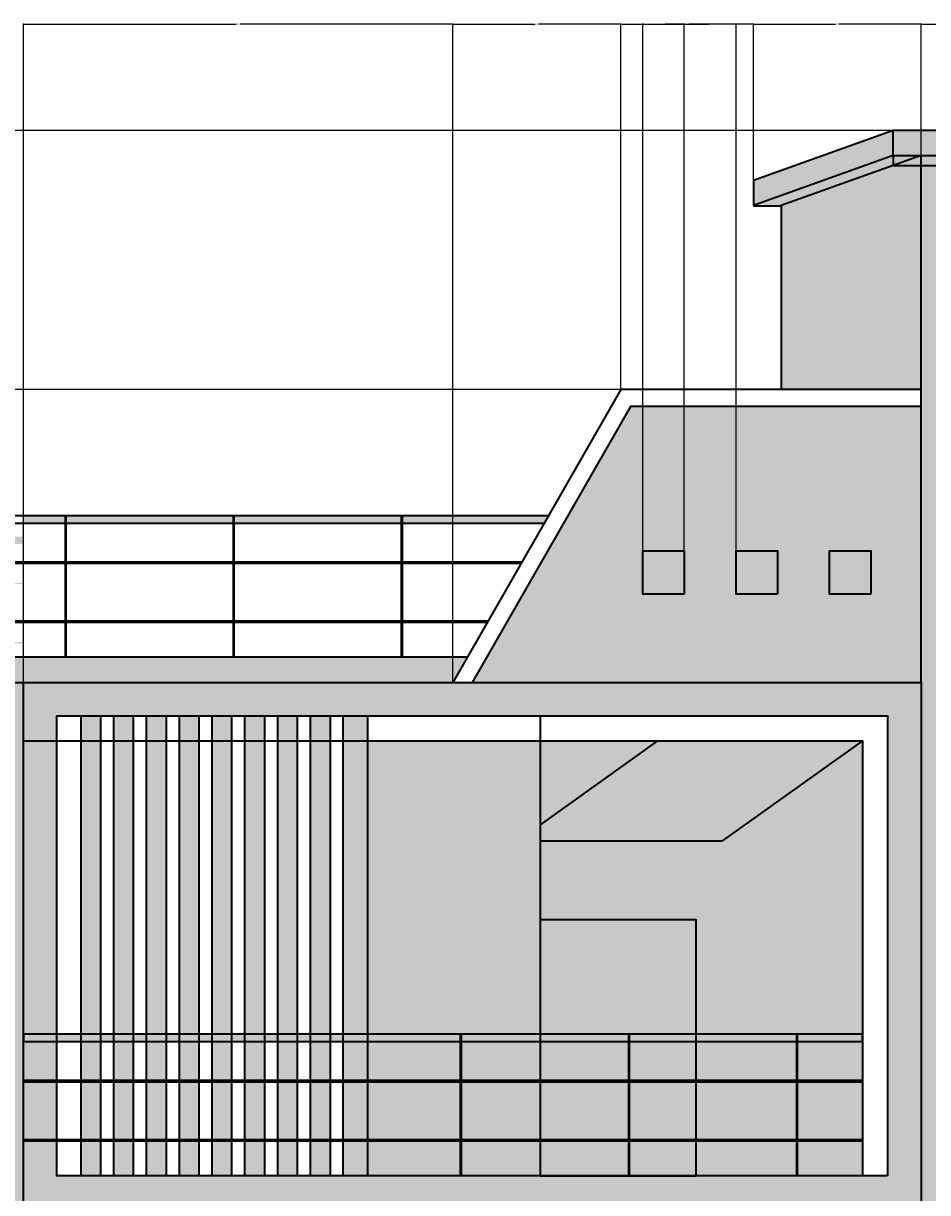
# Model space of a CAD drawing. Units: feet. Extents: x 2415 to 6174, y 866 to 1295.
# Tile 3 of 9: x 3364 to 3580, y 1016 to 1295. Entities that reach past the tile are written whole.
import ezdxf

# ---------------------------------------------------------------- set-up
doc = ezdxf.new("R2010")
doc.units = ezdxf.units.FT
for name, color, linetype, lineweight in [('A-ANNO-DIMS', 2, 'Continuous', 18), ('A-ELEV', 7, 'Continuous', 35), ('A-ELEV-PATT', 8, 'Continuous', 13)]:
    doc.layers.add(name, color=color, linetype=linetype, lineweight=lineweight)
doc.styles.get("Standard").update_dxf_attribs({"font": 'arial.ttf'})
doc.dimstyles.get("Standard").update_dxf_attribs({"dimtxt": 0.18, "dimasz": 0.18, "dimexe": 0.18, "dimexo": 0.0625, "dimgap": 0.09, "dimtad": 0, "dimtih": 1, "dimtoh": 1, "dimdec": 1, "dimzin": 0, "dimdsep": 46, "dimlunit": 3, "dimtxsty": 'Standard', "dimcen": 0.09, "dimadec": 0, "dimazin": 0, "dimtfac": 1, "dimtdec": 1, "dimtofl": 0, "dimtmove": 0, "dimatfit": 3, "dimfxl": 1, "dimtolj": 1, "dimtzin": 0, "dimarcsym": 0})

# ---------------------------------------------------------------- blocks, each defined once
blk = doc.blocks.new('*D63')
at = {"layer": 'A-ANNO-DIMS', "color": 0, "lineweight": -2, "transparency": 16777216}
for p, q in [((3363.87, 1137.66), (3363.87, 1295.18)), ((3364.05, 1295), (3414.78, 1295)), ((3466.42, 1295), (3415.69, 1295)), ((3466.6, 1137.66), (3466.6, 1295.18))]:
    blk.add_line(p, q, dxfattribs=at)
at = {"layer": 'A-ANNO-DIMS', "color": 0, "transparency": 16777216}
for points in [[(3364.05, 1295.03), (3364.05, 1294.97), (3363.87, 1295)], [(3466.42, 1295.03), (3466.42, 1294.97), (3466.6, 1295)]]:
    blk.add_solid(points, dxfattribs=at)
at = {"layer": 'Defpoints', "color": 0, "transparency": 16777216}
for p in [(3466.6, 1295), (3363.87, 1137.6), (3466.6, 1137.6)]:
    blk.add_point(p, dxfattribs=at)
at = {"layer": 'A-ANNO-DIMS', "color": 0, "transparency": 16777216, "insert": (3415.23, 1295), "char_height": 0.18, "attachment_point": 5}
blk.add_mtext('\\A1;102.73', dxfattribs=at)
blk = doc.blocks.new('*D64')
at = {"layer": 'A-ANNO-DIMS', "color": 0, "lineweight": -2, "transparency": 16777216}
for p, q in [((3466.6, 1137.66), (3466.6, 1295.18)), ((3466.78, 1295), (3486.3, 1295)), ((3506.61, 1295), (3487.09, 1295)), ((3506.79, 1207.66), (3506.79, 1295.18))]:
    blk.add_line(p, q, dxfattribs=at)
at = {"layer": 'A-ANNO-DIMS', "color": 0, "transparency": 16777216}
for points in [[(3466.78, 1295.03), (3466.78, 1294.97), (3466.6, 1295)], [(3506.61, 1295.03), (3506.61, 1294.97), (3506.79, 1295)]]:
    blk.add_solid(points, dxfattribs=at)
at = {"layer": 'Defpoints', "color": 0, "transparency": 16777216}
for p in [(3506.79, 1295), (3506.79, 1207.6), (3466.6, 1137.6)]:
    blk.add_point(p, dxfattribs=at)
at = {"layer": 'A-ANNO-DIMS', "color": 0, "transparency": 16777216, "insert": (3486.7, 1295), "char_height": 0.18, "attachment_point": 5}
blk.add_mtext('\\A1;40.19', dxfattribs=at)
blk = doc.blocks.new('*D65')
at = {"layer": 'A-ANNO-DIMS', "color": 0, "lineweight": -2, "transparency": 16777216}
for p, q in [((3506.79, 1207.66), (3506.79, 1295.18)), ((3506.97, 1295), (3522.26, 1295)), ((3538.33, 1295), (3523.04, 1295)), ((3538.51, 1257.71), (3538.51, 1295.18))]:
    blk.add_line(p, q, dxfattribs=at)
at = {"layer": 'A-ANNO-DIMS', "color": 0, "transparency": 16777216}
for points in [[(3506.97, 1295.03), (3506.97, 1294.97), (3506.79, 1295)], [(3538.33, 1295.03), (3538.33, 1294.97), (3538.51, 1295)]]:
    blk.add_solid(points, dxfattribs=at)
at = {"layer": 'Defpoints', "color": 0, "transparency": 16777216}
for p in [(3538.51, 1295), (3538.51, 1257.64), (3506.79, 1207.6)]:
    blk.add_point(p, dxfattribs=at)
at = {"layer": 'A-ANNO-DIMS', "color": 0, "transparency": 16777216, "insert": (3522.65, 1295), "char_height": 0.18, "attachment_point": 5}
blk.add_mtext('\\A1;31.72', dxfattribs=at)
blk = doc.blocks.new('*D66')
at = {"layer": 'A-ANNO-DIMS', "color": 0, "lineweight": -2, "transparency": 16777216}
for p, q in [((3538.51, 1257.71), (3538.51, 1295.18)), ((3538.69, 1295), (3558.07, 1295)), ((3578.38, 1295), (3559, 1295)), ((3578.56, 1263.66), (3578.56, 1295.18))]:
    blk.add_line(p, q, dxfattribs=at)
at = {"layer": 'A-ANNO-DIMS', "color": 0, "transparency": 16777216}
for points in [[(3538.69, 1295.03), (3538.69, 1294.97), (3538.51, 1295)], [(3578.38, 1295.03), (3578.38, 1294.97), (3578.56, 1295)]]:
    blk.add_solid(points, dxfattribs=at)
at = {"layer": 'Defpoints', "color": 0, "transparency": 16777216}
for p in [(3578.56, 1295), (3578.56, 1263.6), (3538.51, 1257.64)]:
    blk.add_point(p, dxfattribs=at)
at = {"layer": 'A-ANNO-DIMS', "color": 0, "transparency": 16777216, "insert": (3558.54, 1295), "char_height": 0.18, "attachment_point": 5}
blk.add_mtext('\\A1;40.046', dxfattribs=at)
blk = doc.blocks.new('*D67')
at = {"layer": 'A-ANNO-DIMS', "color": 0, "lineweight": -2, "transparency": 16777216}
for p, q in [((3578.56, 1263.66), (3578.56, 1295.18)), ((3578.74, 1295), (3589.92, 1295)), ((3602.04, 1295), (3590.85, 1295)), ((3602.22, 1239.13), (3602.22, 1295.18))]:
    blk.add_line(p, q, dxfattribs=at)
at = {"layer": 'A-ANNO-DIMS', "color": 0, "transparency": 16777216}
for points in [[(3578.74, 1295.03), (3578.74, 1294.97), (3578.56, 1295)], [(3602.04, 1295.03), (3602.04, 1294.97), (3602.22, 1295)]]:
    blk.add_solid(points, dxfattribs=at)
at = {"layer": 'Defpoints', "color": 0, "transparency": 16777216}
for p in [(3602.22, 1295), (3578.56, 1263.6), (3602.22, 1239.07)]:
    blk.add_point(p, dxfattribs=at)
at = {"layer": 'A-ANNO-DIMS', "color": 0, "transparency": 16777216, "insert": (3590.39, 1295), "char_height": 0.18, "attachment_point": 5}
blk.add_mtext('\\A1;23.657', dxfattribs=at)
blk = doc.blocks.new('*D77')
at = {"layer": 'A-ANNO-DIMS', "color": 0, "lineweight": -2, "transparency": 16777216}
for p, q in [((3506.73, 1207.6), (3227.55, 1207.6)), ((3227.73, 1207.42), (3227.73, 1192.55)), ((3227.73, 1177.32), (3227.73, 1192.19)), ((3253.07, 1177.14), (3227.55, 1177.14))]:
    blk.add_line(p, q, dxfattribs=at)
at = {"layer": 'A-ANNO-DIMS', "color": 0, "transparency": 16777216}
for points in [[(3227.7, 1207.42), (3227.76, 1207.42), (3227.73, 1207.6)], [(3227.7, 1177.32), (3227.76, 1177.32), (3227.73, 1177.14)]]:
    blk.add_solid(points, dxfattribs=at)
at = {"layer": 'Defpoints', "color": 0, "transparency": 16777216}
for p in [(3227.73, 1207.6), (3506.79, 1207.6), (3253.13, 1177.14)]:
    blk.add_point(p, dxfattribs=at)
at = {"layer": 'A-ANNO-DIMS', "color": 0, "transparency": 16777216, "insert": (3227.73, 1192.37), "char_height": 0.18, "attachment_point": 5}
blk.add_mtext('\\A1;30.457', dxfattribs=at)
blk = doc.blocks.new('*D78')
at = {"layer": 'A-ANNO-DIMS', "color": 0, "lineweight": -2, "transparency": 16777216}
for p, q in [((3571.87, 1269.6), (3227.55, 1269.6)), ((3227.73, 1269.42), (3227.73, 1238.78)), ((3227.73, 1207.78), (3227.73, 1238.42)), ((3506.73, 1207.6), (3227.55, 1207.6))]:
    blk.add_line(p, q, dxfattribs=at)
at = {"layer": 'A-ANNO-DIMS', "color": 0, "transparency": 16777216}
for points in [[(3227.7, 1269.42), (3227.76, 1269.42), (3227.73, 1269.6)], [(3227.7, 1207.78), (3227.76, 1207.78), (3227.73, 1207.6)]]:
    blk.add_solid(points, dxfattribs=at)
at = {"layer": 'Defpoints', "color": 0, "transparency": 16777216}
for p in [(3227.73, 1269.6), (3571.93, 1269.6), (3506.79, 1207.6)]:
    blk.add_point(p, dxfattribs=at)
at = {"layer": 'A-ANNO-DIMS', "color": 0, "transparency": 16777216, "insert": (3227.73, 1238.6), "char_height": 0.18, "attachment_point": 5}
blk.add_mtext('\\A1;62', dxfattribs=at)
blk = doc.blocks.new('*D90')
at = {"layer": 'A-ANNO-DIMS', "color": 0, "lineweight": -2, "transparency": 16777216}
for p, q in [((3512.05, 1169.09), (3512.05, 1295.18)), ((3512.23, 1295), (3516.6, 1295)), ((3521.76, 1295), (3517.39, 1295)), ((3521.94, 1169.09), (3521.94, 1295.18))]:
    blk.add_line(p, q, dxfattribs=at)
at = {"layer": 'A-ANNO-DIMS', "color": 0, "transparency": 16777216}
for points in [[(3512.23, 1295.03), (3512.23, 1294.97), (3512.05, 1295)], [(3521.76, 1295.03), (3521.76, 1294.97), (3521.94, 1295)]]:
    blk.add_solid(points, dxfattribs=at)
at = {"layer": 'Defpoints', "color": 0, "transparency": 16777216}
for p in [(3521.94, 1295), (3512.05, 1169.03), (3521.94, 1169.03)]:
    blk.add_point(p, dxfattribs=at)
at = {"layer": 'A-ANNO-DIMS', "color": 0, "transparency": 16777216, "insert": (3516.99, 1295), "char_height": 0.18, "attachment_point": 5}
blk.add_mtext('\\A1;9.886', dxfattribs=at)
blk = doc.blocks.new('*D91')
at = {"layer": 'A-ANNO-DIMS', "color": 0, "lineweight": -2, "transparency": 16777216}
for p, q in [((3521.94, 1158.74), (3521.94, 1295.18)), ((3522.12, 1295), (3527.7, 1295)), ((3534.2, 1295), (3528.61, 1295)), ((3534.38, 1158.74), (3534.38, 1295.18))]:
    blk.add_line(p, q, dxfattribs=at)
at = {"layer": 'A-ANNO-DIMS', "color": 0, "transparency": 16777216}
for points in [[(3522.12, 1295.03), (3522.12, 1294.97), (3521.94, 1295)], [(3534.2, 1295.03), (3534.2, 1294.97), (3534.38, 1295)]]:
    blk.add_solid(points, dxfattribs=at)
at = {"layer": 'Defpoints', "color": 0, "transparency": 16777216}
for p in [(3534.38, 1295), (3521.94, 1158.67), (3534.38, 1158.67)]:
    blk.add_point(p, dxfattribs=at)
at = {"layer": 'A-ANNO-DIMS', "color": 0, "transparency": 16777216, "insert": (3528.16, 1295), "char_height": 0.18, "attachment_point": 5}
blk.add_mtext('\\A1;12.438', dxfattribs=at)

msp = doc.modelspace()

# ---------------------------------------------------------------- hatches: boundary and pattern name
at = {"layer": 'A-ELEV-PATT'}
h = msp.add_hatch(color=256, dxfattribs=at)
h.set_gradient(color1=(255, 255, 255), tint=1)
h.paths.add_polyline_path([(3264.916, 1143.5993), (3253.129, 1143.5993), (3253.129, 891.5993), (3264.916, 891.5993)])
h.paths.add_polyline_path([(3470.0448, 1143.5993), (3264.916, 1143.5993), (3264.916, 1137.5992), (3466.5999, 1137.5992)])
h.paths.add_polyline_path([(3363.8667, 1137.5992), (3264.916, 1137.5992), (3264.916, 1011.5993), (3363.8667, 1011.5993)])
h.paths.add_polyline_path([(3286.0429, 1117.0591), (3337.7904, 1117.0591), (3337.7904, 1115.4381), (3336.5314, 1115.4381), (3336.5314, 1110.528), (3335.4882, 1110.528), (3335.4882, 1042.3194), (3288.3452, 1042.3194), (3288.3452, 1110.528), (3287.3019, 1110.528), (3287.3019, 1115.4381), (3286.0429, 1115.4381)], flags=16)
h.paths.add_polyline_path([(3290.3452, 1108.528), (3333.4882, 1108.528), (3333.4882, 1044.3194), (3290.3452, 1044.3194)], flags=0)
h.paths.add_polyline_path([(3292.3452, 1106.528), (3331.4882, 1106.528), (3331.4882, 1046.3194), (3292.3452, 1046.3194)], flags=0)
h.paths.add_polyline_path([(3311.7156, 1106.528), (3312.1178, 1106.528), (3312.1178, 1046.3194), (3311.7156, 1046.3194)], flags=0)
h.paths.add_polyline_path([(3682.0722, 1263.5992), (3578.5579, 1263.5992), (3578.5579, 1137.5992), (3578.5579, 961.3655), (3682.0722, 961.3655)])
h.paths.add_polyline_path([(3660.8129, 1239.0671), (3660.8129, 996.6447), (3602.2151, 996.6447), (3602.2151, 1239.0671)], flags=16)
h.paths.add_polyline_path([(3632.2447, 1239.0671), (3632.2447, 996.6447), (3630.7833, 996.6447), (3630.7833, 1029.3019), (3602.2151, 1029.3019), (3602.2151, 1030.7632), (3630.7833, 1030.7632), (3630.7833, 1071.2549), (3602.2151, 1071.2549), (3602.2151, 1072.7163), (3630.7833, 1072.7163), (3630.7833, 1113.2079), (3602.2151, 1113.2079), (3602.2151, 1114.6693), (3630.7833, 1114.6693), (3630.7833, 1155.161), (3602.2151, 1155.161), (3602.2151, 1156.6224), (3630.7833, 1156.6224), (3630.7833, 1197.114), (3602.2151, 1197.114), (3602.2151, 1198.5754), (3630.7833, 1198.5754), (3630.7833, 1239.0671)], flags=0)
h.paths.add_polyline_path([(3733.129, 951.5993), (3634.5374, 951.5993), (3634.5374, 891.5993), (3733.129, 891.5993)])
h.paths.add_polyline_path([(3627.8799, 951.5993), (3621.0953, 951.5993), (3621.0953, 891.5993), (3627.8799, 891.5993)])
h.paths.add_polyline_path([(3614.4378, 951.5993), (3607.6532, 951.5993), (3607.6532, 891.5993), (3614.4378, 891.5993)])
h.paths.add_polyline_path([(3565.9347, 951.5993), (3441.3079, 951.5993), (3441.3079, 891.5993), (3565.9347, 891.5993)], flags=17)
h.paths.add_polyline_path([(3571.9347, 957.5993), (3435.3079, 957.5993), (3435.3079, 891.5993), (3441.3079, 891.5993), (3441.3079, 951.5993), (3565.9347, 951.5993), (3565.9347, 891.5993), (3571.9347, 891.5993)])
h.paths.add_polyline_path([(3435.3079, 1011.5993), (3423.5209, 1011.5993), (3423.5209, 891.5993), (3435.3079, 891.5993), (3435.3079, 957.5993)])
h.paths.add_polyline_path([(3690.0912, 1269.5992), (3571.9347, 1269.5992), (3571.9347, 1263.5992), (3690.0912, 1263.5992)])
h.paths.add_polyline_path([(3571.9347, 1269.5992), (3538.5122, 1257.6449), (3538.5122, 1251.6449), (3571.9347, 1263.5992)])
h = msp.add_hatch(color=256, dxfattribs=at)
h.set_gradient(color1=(205, 105, 40), color2=(205, 105, 40))
h.paths.add_polyline_path([(3682.0722, 1263.5992), (3578.5579, 1263.5992), (3578.5579, 1261.2323), (3682.0722, 1261.2628)])
h.paths.add_polyline_path([(3571.9347, 1261.2303), (3571.9347, 1263.5992), (3538.5122, 1251.6449), (3538.5466, 1251.5295), (3544.7493, 1251.5295), (3545.1353, 1251.6449)])
h.paths.add_polyline_path([(3578.5579, 1263.5992), (3571.9347, 1263.5992), (3571.9347, 1261.2303)])
h.paths.add_polyline_path([(3690.0912, 1263.5992), (3682.0722, 1263.5992), (3682.0722, 1261.2628), (3682.0722, 1259.8122)])
h = msp.add_hatch(color=256, dxfattribs=at)
h.set_gradient(color1=(255, 255, 255))
h.paths.add_polyline_path([(3578.5579, 1263.5992), (3545.1353, 1251.6449), (3545.1353, 1207.5992), (3578.5579, 1207.5992)])
h = msp.add_hatch(color=256, dxfattribs=at)
h.set_gradient(color1=(205, 105, 40), color2=(205, 105, 40))
h.paths.add_polyline_path([(3578.5579, 1263.5992), (3571.9347, 1261.2303), (3578.5579, 1261.2323)])
h = msp.add_hatch(color=256, dxfattribs=at)
h.set_gradient(color1=(205, 105, 40), color2=(205, 105, 40))
h.paths.add_polyline_path([(3578.5579, 1203.5993), (3509.1068, 1203.5993), (3471.2123, 1137.5992), (3578.5579, 1137.5992)])
h.paths.add_polyline_path([(3521.9379, 1169.0289), (3521.9379, 1158.6726), (3512.0517, 1158.6726), (3512.0517, 1169.0289)], flags=16)
h.paths.add_polyline_path([(3534.3754, 1169.0289), (3544.2616, 1169.0289), (3544.2616, 1158.6726), (3534.3754, 1158.6726)], flags=16)
h.paths.add_polyline_path([(3556.6991, 1169.0289), (3566.5853, 1169.0289), (3566.5853, 1158.6726), (3556.6991, 1158.6726)], flags=16)
h.paths.add_polyline_path([(3687.1301, 1136.3701), (3684.8039, 1136.3701), (3684.8039, 1030.9315), (3687.1301, 1030.9315)])
h.paths.add_polyline_path([(3692.5646, 1136.3701), (3690.2384, 1136.3701), (3690.2384, 1030.9315), (3692.5646, 1030.9315)])
h.paths.add_polyline_path([(3697.9991, 1136.3701), (3695.6729, 1136.3701), (3695.6729, 1030.9315), (3697.9991, 1030.9315)])
h.paths.add_polyline_path([(3703.4336, 1136.3701), (3701.1074, 1136.3701), (3701.1074, 1030.9315), (3703.4336, 1030.9315)])
h.paths.add_polyline_path([(3708.8681, 1136.3701), (3706.5419, 1136.3701), (3706.5419, 1030.9315), (3708.8681, 1030.9315)])
h.paths.add_polyline_path([(3714.3026, 1136.3701), (3711.9764, 1136.3701), (3711.9764, 1030.9315), (3714.3026, 1030.9315)])
h.paths.add_polyline_path([(3719.7371, 1136.3701), (3717.4109, 1136.3701), (3717.4109, 1030.9315), (3719.7371, 1030.9315)])
h.paths.add_polyline_path([(3725.1716, 1136.3701), (3722.8454, 1136.3701), (3722.8454, 1030.9315), (3725.1716, 1030.9315)])
h.paths.add_polyline_path([(3730.6061, 1136.3701), (3728.2799, 1136.3701), (3728.2799, 1030.9315), (3730.6061, 1030.9315)])
h.paths.add_polyline_path([(3382.3104, 1123.5993), (3377.658, 1123.5993), (3377.658, 1053.4585), (3382.3104, 1053.4585)], flags=17)
h.paths.add_polyline_path([(3390.153, 1123.5993), (3385.5006, 1123.5993), (3385.5006, 1053.4585), (3390.153, 1053.4585)], flags=17)
h.paths.add_polyline_path([(3382.3104, 1129.5993), (3377.658, 1129.5993), (3377.658, 1123.5993), (3382.3104, 1123.5993)], flags=17)
h.paths.add_polyline_path([(3390.153, 1129.5993), (3385.5006, 1129.5993), (3385.5006, 1123.5993), (3390.153, 1123.5993)], flags=17)
h.paths.add_polyline_path([(3397.9956, 1129.5993), (3393.3432, 1129.5993), (3393.3432, 1123.5993), (3397.9956, 1123.5993)])
h.paths.add_polyline_path([(3397.9956, 1123.5993), (3393.3432, 1123.5993), (3393.3432, 1019.5993), (3397.9956, 1019.5993)])
h.paths.add_polyline_path([(3405.8382, 1129.5993), (3401.1858, 1129.5993), (3401.1858, 1123.5993), (3405.8382, 1123.5993)])
h.paths.add_polyline_path([(3405.8382, 1123.5993), (3401.1858, 1123.5993), (3401.1858, 1019.5993), (3405.8382, 1019.5993)])
h.paths.add_polyline_path([(3413.6808, 1129.5993), (3409.0284, 1129.5993), (3409.0284, 1123.5993), (3413.6808, 1123.5993)])
h.paths.add_polyline_path([(3413.6808, 1123.5993), (3409.0284, 1123.5993), (3409.0284, 1019.5993), (3413.6808, 1019.5993)])
h.paths.add_polyline_path([(3421.5234, 1129.5993), (3416.871, 1129.5993), (3416.871, 1123.5993), (3421.5234, 1123.5993)])
h.paths.add_polyline_path([(3421.5234, 1123.5993), (3416.871, 1123.5993), (3416.871, 1019.5993), (3421.5234, 1019.5993)])
h.paths.add_polyline_path([(3429.366, 1129.5993), (3424.7136, 1129.5993), (3424.7136, 1123.5993), (3429.366, 1123.5993)])
h.paths.add_polyline_path([(3429.366, 1123.5993), (3424.7136, 1123.5993), (3424.7136, 1019.5993), (3429.366, 1019.5993)])
h.paths.add_polyline_path([(3437.2086, 1129.5993), (3432.5562, 1129.5993), (3432.5562, 1123.5993), (3437.2086, 1123.5993)])
h.paths.add_polyline_path([(3437.2086, 1123.5993), (3432.5562, 1123.5993), (3432.5562, 1019.5993), (3437.2086, 1019.5993)])
h.paths.add_polyline_path([(3446.1534, 1129.5993), (3440.3202, 1129.5993), (3440.3202, 1123.5993), (3446.1534, 1123.5993)])
h.paths.add_polyline_path([(3446.1534, 1123.5993), (3440.3202, 1123.5993), (3440.3202, 1019.5993), (3446.1534, 1019.5993)])
h.paths.add_polyline_path([(3390.153, 1123.5993), (3385.5006, 1123.5993), (3385.5006, 1053.4585), (3385.5006, 1019.5993), (3390.153, 1019.5993)])
h.paths.add_polyline_path([(3390.153, 1123.5993), (3390.153, 1129.5993), (3385.5006, 1129.5993), (3385.5006, 1053.4585), (3390.153, 1053.4585)])
h.paths.add_polyline_path([(3382.3104, 1027.963), (3377.658, 1027.963), (3377.658, 1019.5993), (3382.3104, 1019.5993)])
h.paths.add_polyline_path([(3382.3104, 1028.2269), (3377.658, 1028.2269), (3377.658, 1027.963), (3382.3104, 1027.963)])
h.paths.add_polyline_path([(3382.3104, 1129.5993), (3377.658, 1129.5993), (3377.658, 1028.2269), (3382.3104, 1028.2269)])
h = msp.add_hatch(color=256, dxfattribs=at)
h.set_gradient(color2=(0, 0, 0))
h.paths.add_polyline_path([(3489.4854, 1177.4585), (3454.5146, 1177.4585), (3454.5146, 1175.7117), (3488.4825, 1175.7117)])
h.paths.add_polyline_path([(3454.5146, 1177.4585), (3454.2507, 1177.4585), (3454.2507, 1175.7117), (3454.5146, 1175.7117)])
h.paths.add_polyline_path([(3454.5146, 1175.7117), (3454.2507, 1175.7117), (3454.2507, 1166.3873), (3454.5146, 1166.3873)])
h.paths.add_polyline_path([(3454.5146, 1166.3873), (3454.2507, 1166.3873), (3454.2507, 1166.1234), (3454.5146, 1166.1234)])
h.paths.add_polyline_path([(3483.1288, 1166.3873), (3454.5146, 1166.3873), (3454.5146, 1166.1234), (3482.9773, 1166.1234)])
h.paths.add_polyline_path([(3454.2507, 1166.3873), (3414.3148, 1166.3873), (3414.3148, 1166.1234), (3454.2507, 1166.1234)])
h.paths.add_polyline_path([(3454.5146, 1166.1234), (3454.2507, 1166.1234), (3454.2507, 1152.2269), (3454.5146, 1152.2269)])
h.paths.add_polyline_path([(3454.5146, 1152.2269), (3454.2507, 1152.2269), (3454.2507, 1151.963), (3454.5146, 1151.963)])
h.paths.add_polyline_path([(3474.9985, 1152.2269), (3454.5146, 1152.2269), (3454.5146, 1151.963), (3474.8469, 1151.963)])
h.paths.add_polyline_path([(3454.2507, 1152.2269), (3414.3148, 1152.2269), (3414.3148, 1151.963), (3454.2507, 1151.963)])
h.paths.add_polyline_path([(3454.5146, 1151.963), (3454.2507, 1151.963), (3454.2507, 1143.5993), (3454.5146, 1143.5993)])
h.paths.add_polyline_path([(3414.3148, 1175.7117), (3414.0509, 1175.7117), (3414.0509, 1166.3873), (3414.3148, 1166.3873)])
h.paths.add_polyline_path([(3414.3148, 1166.1234), (3414.0509, 1166.1234), (3414.0509, 1152.2269), (3414.3148, 1152.2269)])
h.paths.add_polyline_path([(3414.3148, 1152.2269), (3414.0509, 1152.2269), (3414.0509, 1151.963), (3414.3148, 1151.963)])
h.paths.add_polyline_path([(3414.3148, 1151.963), (3414.0509, 1151.963), (3414.0509, 1143.5993), (3414.3148, 1143.5993)])
h.paths.add_polyline_path([(3414.0509, 1152.2269), (3374.115, 1152.2269), (3374.115, 1151.963), (3414.0509, 1151.963)])
h.paths.add_polyline_path([(3374.115, 1166.1234), (3373.851, 1166.1234), (3373.851, 1152.2269), (3374.115, 1152.2269)])
h.paths.add_polyline_path([(3374.115, 1151.963), (3373.851, 1151.963), (3373.851, 1143.5993), (3374.115, 1143.5993)])
h.paths.add_polyline_path([(3363.6028, 1172.4585), (3333.9151, 1172.4585), (3333.9151, 1170.7117), (3363.6028, 1170.7117)])
h.paths.add_polyline_path([(3293.4514, 1172.4585), (3253.5155, 1172.4585), (3253.5155, 1171.8725), (3254.2811, 1170.7117), (3293.4514, 1170.7117)])
h.paths.add_polyline_path([(3333.6512, 1172.4585), (3293.7153, 1172.4585), (3293.7153, 1170.7117), (3333.6512, 1170.7117)])
h.paths.add_polyline_path([(3293.7153, 1172.4585), (3293.4514, 1172.4585), (3293.4514, 1170.7117), (3293.7153, 1170.7117)])
h.paths.add_polyline_path([(3333.9151, 1172.4585), (3333.6512, 1172.4585), (3333.6512, 1170.7117), (3333.9151, 1170.7117)])
h.paths.add_polyline_path([(3333.9151, 1170.7117), (3333.6512, 1170.7117), (3333.6512, 1161.3873), (3333.9151, 1161.3873)])
h.paths.add_polyline_path([(3333.9151, 1161.3873), (3333.6512, 1161.3873), (3333.6512, 1161.1234), (3333.9151, 1161.1234)])
h.paths.add_polyline_path([(3363.6028, 1161.3873), (3333.9151, 1161.3873), (3333.9151, 1161.1234), (3363.6028, 1161.1234)])
h.paths.add_polyline_path([(3333.6512, 1161.3873), (3293.7153, 1161.3873), (3293.7153, 1161.1234), (3333.6512, 1161.1234)])
h.paths.add_polyline_path([(3333.9151, 1161.1234), (3333.6512, 1161.1234), (3333.6512, 1147.2269), (3333.9151, 1147.2269)])
h.paths.add_polyline_path([(3333.9151, 1147.2269), (3333.6512, 1147.2269), (3333.6512, 1146.963), (3333.9151, 1146.963)])
h.paths.add_polyline_path([(3333.9151, 1146.963), (3333.6512, 1146.963), (3333.6512, 1143.5993), (3333.9151, 1143.5993)])
h.paths.add_polyline_path([(3363.6028, 1147.2269), (3333.9151, 1147.2269), (3333.9151, 1146.963), (3363.6028, 1146.963)])
h.paths.add_polyline_path([(3333.6512, 1147.2269), (3293.7153, 1147.2269), (3293.7153, 1146.963), (3333.6512, 1146.963)])
h.paths.add_polyline_path([(3293.7153, 1170.7117), (3293.4514, 1170.7117), (3293.4514, 1161.3873), (3293.7153, 1161.3873)])
h.paths.add_polyline_path([(3293.7153, 1161.1234), (3293.4514, 1161.1234), (3293.4514, 1147.2269), (3293.7153, 1147.2269)])
h.paths.add_polyline_path([(3293.7153, 1161.3873), (3293.4514, 1161.3873), (3293.4514, 1161.1234), (3293.7153, 1161.1234)])
h.paths.add_polyline_path([(3293.4514, 1161.3873), (3260.4316, 1161.3873), (3260.6056, 1161.1234), (3293.4514, 1161.1234)])
h.paths.add_polyline_path([(3293.7153, 1147.2269), (3293.4514, 1147.2269), (3293.4514, 1146.963), (3293.7153, 1146.963)])
h.paths.add_polyline_path([(3293.7153, 1146.963), (3293.4514, 1146.963), (3293.4514, 1143.5993), (3293.7153, 1143.5993)])
h.paths.add_polyline_path([(3293.4514, 1147.2269), (3269.7719, 1147.2269), (3269.946, 1146.963), (3293.4514, 1146.963)])
h.paths.add_polyline_path([(3254.2811, 1170.7117), (3253.5155, 1170.7117), (3253.5155, 1168.7002), (3258.3391, 1161.3873), (3260.4316, 1161.3873)])
h.paths.add_polyline_path([(3260.4316, 1161.3873), (3258.3391, 1161.3873), (3258.5131, 1161.1234), (3260.6056, 1161.1234)])
h.paths.add_polyline_path([(3260.6056, 1161.1234), (3258.5131, 1161.1234), (3267.6794, 1147.2269), (3269.7719, 1147.2269)])
h.paths.add_polyline_path([(3258.3391, 1161.3873), (3253.5155, 1161.3873), (3253.5155, 1161.1234), (3258.5131, 1161.1234)])
h.paths.add_polyline_path([(3269.7719, 1147.2269), (3267.6794, 1147.2269), (3267.8535, 1146.963), (3269.946, 1146.963)])
h.paths.add_polyline_path([(3269.946, 1146.963), (3267.8535, 1146.963), (3270.0722, 1143.5993), (3272.1647, 1143.5993)])
h.paths.add_polyline_path([(3267.6794, 1147.2269), (3256.5092, 1147.2269), (3256.6833, 1146.963), (3267.8535, 1146.963)])
h.paths.add_polyline_path([(3256.1931, 1147.2269), (3253.5155, 1147.2269), (3253.5155, 1146.963), (3256.3671, 1146.963)])
h.paths.add_polyline_path([(3253.5155, 1151.7656), (3253.5155, 1151.2863), (3256.1931, 1147.2269), (3256.5092, 1147.2269)])
h.paths.add_polyline_path([(3256.5092, 1147.2269), (3256.1931, 1147.2269), (3256.3671, 1146.963), (3256.6833, 1146.963)])
h.paths.add_polyline_path([(3256.6833, 1146.963), (3256.3671, 1146.963), (3258.5859, 1143.5993), (3258.902, 1143.5993)])
h.paths.add_polyline_path([(3253.2515, 1152.1657), (3253.2515, 1151.6864), (3253.5155, 1151.2863), (3253.5155, 1151.7656)])
h.paths.add_polyline_path([(3253.5155, 1168.7002), (3253.2515, 1169.1003), (3253.2515, 1152.1657), (3253.5155, 1151.7656)])
h.paths.add_polyline_path([(3253.5155, 1151.2863), (3253.2515, 1151.6864), (3253.2515, 1147.2269), (3253.5155, 1147.2269)])
h.paths.add_polyline_path([(3253.5155, 1147.2269), (3253.2515, 1147.2269), (3253.2515, 1146.963), (3253.5155, 1146.963)])
h.paths.add_polyline_path([(3253.5155, 1146.963), (3253.2515, 1146.963), (3253.2515, 1143.5993), (3253.5155, 1143.5993)])
h.paths.add_polyline_path([(3253.5155, 1171.8725), (3253.2515, 1172.2726), (3253.2515, 1169.1003), (3253.5155, 1168.7002)])
h.paths.add_polyline_path([(3253.5155, 1172.4585), (3253.2515, 1172.4585), (3253.2515, 1172.2726), (3253.5155, 1171.8725)])
h.paths.add_polyline_path([(3253.5155, 1171.8725), (3253.5155, 1170.7117), (3254.2811, 1170.7117)], flags=17)
h.paths.add_polyline_path([(3692.5426, 1181.1411), (3682.0722, 1181.1411), (3682.0722, 1179.3943), (3692.5426, 1179.3943)])
h.paths.add_polyline_path([(3732.7425, 1180.5551), (3732.7425, 1181.1411), (3692.8065, 1181.1411), (3692.8065, 1179.3943), (3731.9768, 1179.3943)])
h.paths.add_polyline_path([(3692.8065, 1181.1411), (3692.5426, 1181.1411), (3692.5426, 1179.3943), (3692.8065, 1179.3943)])
h.paths.add_polyline_path([(3692.8065, 1179.3943), (3692.5426, 1179.3943), (3692.5426, 1170.0699), (3692.8065, 1170.0699)])
h.paths.add_polyline_path([(3725.8264, 1170.0699), (3692.8065, 1170.0699), (3692.8065, 1169.806), (3725.6523, 1169.806)])
h.paths.add_polyline_path([(3692.5426, 1170.0699), (3682.0722, 1170.0699), (3682.0722, 1169.806), (3692.5426, 1169.806)])
h.paths.add_polyline_path([(3692.8065, 1170.0699), (3692.5426, 1170.0699), (3692.5426, 1169.806), (3692.8065, 1169.806)])
h.paths.add_polyline_path([(3692.8065, 1169.806), (3692.5426, 1169.806), (3692.5426, 1156.9315), (3692.8065, 1156.9315)])
h.paths.add_polyline_path([(3733.0064, 1180.9552), (3733.0064, 1181.1411), (3732.7425, 1181.1411), (3732.7425, 1180.5551)])
h.paths.add_polyline_path([(3733.0064, 1180.9058), (3732.9836, 1180.9208), (3732.7425, 1180.5551), (3732.7425, 1179.3943), (3733.0064, 1179.3943)])
h.paths.add_polyline_path([(3732.7425, 1180.5551), (3731.9768, 1179.3943), (3732.7425, 1179.3943)], flags=17)
h.paths.add_polyline_path([(3732.7425, 1179.3943), (3731.9768, 1179.3943), (3725.8264, 1170.0699), (3727.9189, 1170.0699), (3732.7425, 1177.3828)])
h.paths.add_polyline_path([(3733.0064, 1179.3943), (3732.7425, 1179.3943), (3732.7425, 1177.3828), (3733.0064, 1177.7829)])
h.paths.add_polyline_path([(3733.0064, 1170.0699), (3732.7425, 1170.0699), (3732.7425, 1169.806), (3733.0064, 1169.806)])
h.paths.add_polyline_path([(3733.0064, 1177.7829), (3732.7425, 1177.3828), (3732.7425, 1170.0699), (3733.0064, 1170.0699)])
h.paths.add_polyline_path([(3732.7425, 1170.0699), (3727.9189, 1170.0699), (3727.7448, 1169.806), (3732.7425, 1169.806)])
h.paths.add_polyline_path([(3727.9189, 1170.0699), (3725.8264, 1170.0699), (3725.6523, 1169.806), (3727.7448, 1169.806)])
h.paths.add_polyline_path([(3727.7448, 1169.806), (3725.6523, 1169.806), (3717.1602, 1156.9315), (3719.2527, 1156.9315)])
h.paths.add_polyline_path([(3733.0064, 1160.369), (3733.0064, 1160.8483), (3732.7425, 1160.4482), (3732.7425, 1159.9689)])
h.paths.add_polyline_path([(3733.0064, 1169.806), (3732.7425, 1169.806), (3732.7425, 1160.4482), (3733.0064, 1160.8483)])
h.paths.add_polyline_path([(3733.0064, 1160.369), (3732.7425, 1159.9689), (3732.7425, 1156.9315), (3733.0064, 1156.9315)])
h = msp.add_hatch(color=256, dxfattribs=at)
h.set_gradient(color2=(0, 0, 0))
h.paths.add_polyline_path([(3373.851, 1177.4585), (3363.8667, 1177.4585), (3363.8667, 1175.7117), (3373.851, 1175.7117)])
h.paths.add_polyline_path([(3374.115, 1177.4585), (3373.851, 1177.4585), (3373.851, 1175.7117), (3374.115, 1175.7117)])
h.paths.add_polyline_path([(3414.0509, 1177.4585), (3374.115, 1177.4585), (3374.115, 1175.7117), (3414.0509, 1175.7117)])
h.paths.add_polyline_path([(3414.3148, 1177.4585), (3414.0509, 1177.4585), (3414.0509, 1175.7117), (3414.3148, 1175.7117)])
h.paths.add_polyline_path([(3363.8667, 1177.4585), (3363.6028, 1177.4585), (3363.6028, 1172.4585), (3363.8667, 1172.4585)])
h.paths.add_polyline_path([(3363.8667, 1172.4585), (3363.6028, 1172.4585), (3363.6028, 1170.7117), (3363.8667, 1170.7117)])
h.paths.add_polyline_path([(3363.8667, 1170.7117), (3363.6028, 1170.7117), (3363.6028, 1161.3873), (3363.8667, 1161.3873)])
h.paths.add_polyline_path([(3363.8667, 1161.3873), (3363.6028, 1161.3873), (3363.6028, 1161.1234), (3363.8667, 1161.1234)])
h.paths.add_polyline_path([(3363.8667, 1161.1234), (3363.6028, 1161.1234), (3363.6028, 1147.2269), (3363.8667, 1147.2269)])
h.paths.add_polyline_path([(3363.8667, 1147.2269), (3363.6028, 1147.2269), (3363.6028, 1146.963), (3363.8667, 1146.963)])
h.paths.add_polyline_path([(3363.8667, 1146.963), (3363.6028, 1146.963), (3363.6028, 1143.5993), (3363.8667, 1143.5993)])
h.paths.add_polyline_path([(3373.851, 1152.2269), (3363.8667, 1152.2269), (3363.8667, 1151.963), (3373.851, 1151.963)])
h.paths.add_polyline_path([(3374.115, 1152.2269), (3373.851, 1152.2269), (3373.851, 1151.963), (3374.115, 1151.963)])
h.paths.add_polyline_path([(3374.115, 1175.7117), (3373.851, 1175.7117), (3373.851, 1166.3873), (3374.115, 1166.3873)])
h.paths.add_polyline_path([(3373.851, 1166.3873), (3363.8667, 1166.3873), (3363.8667, 1166.1234), (3373.851, 1166.1234)])
h.paths.add_polyline_path([(3374.115, 1166.3873), (3373.851, 1166.3873), (3373.851, 1166.1234), (3374.115, 1166.1234)])
h.paths.add_polyline_path([(3414.0509, 1166.3873), (3374.115, 1166.3873), (3374.115, 1166.1234), (3414.0509, 1166.1234)])
h = msp.add_hatch(color=256, dxfattribs=at)
h.set_gradient(color2=(0, 0, 0))
h.paths.add_polyline_path([(3454.2507, 1177.4585), (3414.3148, 1177.4585), (3414.3148, 1175.7117), (3454.2507, 1175.7117)])
h = msp.add_hatch(color=256, dxfattribs=at)
h.set_gradient(color1=(99, 100, 102), color2=(99, 100, 102))
h.paths.add_polyline_path([(3566.5853, 1169.0289), (3556.6991, 1169.0289), (3556.6991, 1158.6726), (3566.5853, 1158.6726)])
h.paths.add_polyline_path([(3544.2616, 1169.0289), (3534.3754, 1169.0289), (3534.3754, 1158.6726), (3544.2616, 1158.6726)])
h.paths.add_polyline_path([(3521.9379, 1169.0289), (3512.0517, 1169.0289), (3512.0517, 1158.6726), (3521.9379, 1158.6726)])
h = msp.add_hatch(color=256, dxfattribs=at)
h.set_gradient(color1=(99, 100, 102), color2=(99, 100, 102))
h.paths.add_polyline_path([(3578.5579, 1137.5992), (3363.8667, 1137.5992), (3363.8667, 1123.5993), (3371.8667, 1123.5993), (3371.8667, 1129.5993), (3570.5579, 1129.5993), (3570.5579, 1019.5993), (3371.8667, 1019.5993), (3371.8667, 1027.963), (3363.8667, 1027.963), (3363.8667, 1011.5993), (3571.9347, 1011.5993), (3578.5579, 1011.5993)])
h.paths.add_polyline_path([(3371.8667, 1123.5993), (3363.8667, 1123.5993), (3363.8667, 1053.4585), (3371.8667, 1053.4585)], flags=17)
h.paths.add_polyline_path([(3371.8667, 1042.1234), (3363.8667, 1042.1234), (3363.8667, 1028.2269), (3371.8667, 1028.2269)], flags=17)
h.paths.add_polyline_path([(3371.8667, 1051.7117), (3363.8667, 1051.7117), (3363.8667, 1042.3873), (3371.8667, 1042.3873)], flags=17)
h.paths.add_polyline_path([(3371.8667, 1053.4585), (3363.8667, 1053.4585), (3363.8667, 1051.7117), (3371.8667, 1051.7117)], flags=17)
h.paths.add_polyline_path([(3371.8667, 1042.3873), (3363.8667, 1042.3873), (3363.8667, 1042.1234), (3371.8667, 1042.1234)], flags=17)
h.paths.add_polyline_path([(3371.8667, 1028.2269), (3363.8667, 1028.2269), (3363.8667, 1027.963), (3371.8667, 1027.963)], flags=17)
h = msp.add_hatch(color=256, dxfattribs=at)
h.set_gradient(color1=(205, 105, 40), color2=(205, 105, 40))
h.paths.add_polyline_path([(3390.153, 1129.5993), (3385.5006, 1129.5993), (3385.5006, 1123.5993), (3390.153, 1123.5993)])
h.paths.add_polyline_path([(3382.3104, 1129.5993), (3377.658, 1129.5993), (3377.658, 1123.5993), (3382.3104, 1123.5993)])
h.paths.add_polyline_path([(3382.3104, 1123.5993), (3377.658, 1123.5993), (3377.658, 1019.5993), (3382.3104, 1019.5993)])
h = msp.add_hatch(color=256, dxfattribs=at)
h.set_gradient(color1=(248, 246, 176), name='CURVED')
h.paths.add_polyline_path([(3487.443, 1123.5993), (3446.1534, 1123.5993), (3446.1534, 1053.4585), (3487.443, 1053.4585), (3487.443, 1080.8275)])
h.paths.add_polyline_path([(3468.3641, 1051.7117), (3446.1534, 1051.7117), (3446.1534, 1028.2269), (3468.3641, 1028.2269)])
h.paths.add_polyline_path([(3487.443, 1051.7117), (3468.628, 1051.7117), (3468.628, 1028.2269), (3487.443, 1028.2269)])
h.paths.add_polyline_path([(3468.3641, 1027.963), (3446.1534, 1027.963), (3446.1534, 1019.5993), (3468.3641, 1019.5993)])
h.paths.add_polyline_path([(3487.443, 1027.963), (3468.628, 1027.963), (3468.628, 1019.5993), (3487.443, 1019.5993)])
h.paths.add_polyline_path([(3564.5579, 1123.5993), (3530.9457, 1099.6515), (3487.443, 1099.6515), (3487.443, 1080.8275), (3524.8012, 1080.8275), (3524.8012, 1053.4585), (3564.5579, 1053.4585)])
h.paths.add_polyline_path([(3548.7638, 1051.7117), (3524.8012, 1051.7117), (3524.8012, 1028.2269), (3548.7638, 1028.2269)])
h.paths.add_polyline_path([(3548.7638, 1027.963), (3524.8012, 1027.963), (3524.8012, 1019.5993), (3548.7638, 1019.5993)])
h.paths.add_polyline_path([(3564.5579, 1027.963), (3549.0277, 1027.963), (3549.0277, 1019.5993), (3564.5579, 1019.5993)])
h.paths.add_polyline_path([(3388.4421, 1011.5993), (3264.916, 1011.5993), (3264.916, 960.433), (3388.4421, 960.433)])
h.paths.add_polyline_path([(3571.9347, 1011.5993), (3435.3079, 1011.5993), (3435.3079, 957.5993), (3571.9347, 957.5993)])
h.paths.add_polyline_path([(3423.5209, 1011.5993), (3400.3333, 1011.5993), (3400.3333, 960.433), (3423.5209, 960.433)])
h = msp.add_hatch(color=256, dxfattribs=at)
h.set_gradient(color1=(251, 249, 203), color2=(251, 249, 203), name='CURVED')
h.paths.add_polyline_path([(3564.5579, 1123.5993), (3530.9457, 1099.6515), (3487.443, 1099.6515), (3487.443, 1080.8275), (3524.8012, 1080.8275), (3524.8012, 1053.4585), (3564.5579, 1053.4585)])
h.paths.add_polyline_path([(3564.5579, 1123.5993), (3515.549, 1123.5993), (3487.443, 1103.5745), (3487.443, 1099.6515), (3530.9457, 1099.6515)], flags=17)
h.paths.add_polyline_path([(3515.549, 1123.5993), (3487.443, 1123.5993), (3487.443, 1103.5745)], flags=16)
h.paths.add_polyline_path([(3564.5579, 1051.7117), (3549.0277, 1051.7117), (3549.0277, 1028.2269), (3564.5579, 1028.2269)])
h = msp.add_hatch(color=256, dxfattribs=at)
h.set_gradient(color1=(242, 103, 34), color2=(242, 103, 34))
h.paths.add_polyline_path([(3524.8012, 1080.8275), (3487.443, 1080.8275), (3487.443, 1053.4585), (3524.8012, 1053.4585)])
h.paths.add_polyline_path([(3508.5639, 1051.7117), (3487.443, 1051.7117), (3487.443, 1042.3873), (3508.5639, 1042.3873)])
h.paths.add_polyline_path([(3524.8012, 1051.7117), (3508.8278, 1051.7117), (3508.8278, 1042.3873), (3524.8012, 1042.3873)])
h.paths.add_polyline_path([(3524.8012, 1042.1234), (3508.8278, 1042.1234), (3508.8278, 1028.2269), (3524.8012, 1028.2269)])
h.paths.add_polyline_path([(3508.5639, 1042.1234), (3487.443, 1042.1234), (3487.443, 1028.2269), (3508.5639, 1028.2269)])
h.paths.add_polyline_path([(3508.5639, 1027.963), (3487.443, 1027.963), (3487.443, 1019.5993), (3508.5639, 1019.5993)])
h.paths.add_polyline_path([(3524.8012, 1027.963), (3508.8278, 1027.963), (3508.8278, 1019.5993), (3524.8012, 1019.5993)])
h = msp.add_hatch(color=256, dxfattribs=at)
h.set_gradient(color2=(0, 0, 0))
h.paths.add_polyline_path([(3468.3641, 1053.4585), (3371.8667, 1053.4585), (3371.8667, 1051.7117), (3468.3641, 1051.7117)])
h.paths.add_polyline_path([(3468.628, 1053.4585), (3468.3641, 1053.4585), (3468.3641, 1051.7117), (3468.628, 1051.7117)])
h.paths.add_polyline_path([(3564.5579, 1053.4585), (3468.628, 1053.4585), (3468.628, 1051.7117), (3564.5579, 1051.7117)])
h.paths.add_polyline_path([(3549.0277, 1051.7117), (3548.7638, 1051.7117), (3548.7638, 1042.3873), (3549.0277, 1042.3873)])
h.paths.add_polyline_path([(3549.0277, 1042.3873), (3548.7638, 1042.3873), (3548.7638, 1042.1234), (3549.0277, 1042.1234)], flags=16)
h.paths.add_polyline_path([(3564.5579, 1042.3873), (3549.0277, 1042.3873), (3549.0277, 1042.1234), (3564.5579, 1042.1234)], flags=16)
h.paths.add_polyline_path([(3548.7638, 1042.3873), (3508.8278, 1042.3873), (3508.8278, 1042.1234), (3548.7638, 1042.1234)], flags=16)
h.paths.add_polyline_path([(3549.0277, 1042.1234), (3548.7638, 1042.1234), (3548.7638, 1028.2269), (3549.0277, 1028.2269)])
h.paths.add_polyline_path([(3549.0277, 1028.2269), (3548.7638, 1028.2269), (3548.7638, 1027.963), (3549.0277, 1027.963)], flags=16)
h.paths.add_polyline_path([(3549.0277, 1027.963), (3548.7638, 1027.963), (3548.7638, 1019.5993), (3549.0277, 1019.5993)])
h.paths.add_polyline_path([(3564.5579, 1028.2269), (3549.0277, 1028.2269), (3549.0277, 1027.963), (3564.5579, 1027.963)], flags=17)
h.paths.add_polyline_path([(3548.7638, 1028.2269), (3508.8278, 1028.2269), (3508.8278, 1027.963), (3548.7638, 1027.963)], flags=16)
h.paths.add_polyline_path([(3468.628, 1051.7117), (3468.3641, 1051.7117), (3468.3641, 1042.3873), (3468.628, 1042.3873)])
h.paths.add_polyline_path([(3468.628, 1042.3873), (3468.3641, 1042.3873), (3468.3641, 1042.1234), (3468.628, 1042.1234)], flags=16)
h.paths.add_polyline_path([(3564.5579, 1042.3873), (3468.628, 1042.3873), (3468.628, 1042.1234), (3564.5579, 1042.1234)], flags=17)
h.paths.add_polyline_path([(3564.5579, 1028.2269), (3371.8667, 1028.2269), (3371.8667, 1027.963), (3564.5579, 1027.963)])
h.paths.add_polyline_path([(3564.5579, 1042.3873), (3371.8667, 1042.3873), (3371.8667, 1042.1234), (3564.5579, 1042.1234)])
h.paths.add_polyline_path([(3468.628, 1042.1234), (3468.3641, 1042.1234), (3468.3641, 1028.2269), (3468.628, 1028.2269)])
h.paths.add_polyline_path([(3468.628, 1027.963), (3468.3641, 1027.963), (3468.3641, 1019.5993), (3468.628, 1019.5993)])

# ---------------------------------------------------------------- linework, layer by layer
at = {"layer": 'A-ELEV'}
for p, q in [((3571.9347, 1269.5992), (3538.5122, 1257.6449)), ((3690.0912, 1269.5992), (3571.9347, 1269.5992)), ((3571.9347, 1263.5992), (3571.9347, 1269.5992)), ((3571.9347, 1263.5992), (3538.5122, 1251.6449)), ((3578.5579, 1263.5992), (3545.1353, 1251.6449)), ((3571.9347, 1263.5992), (3690.0912, 1263.5992)), ((3571.9347, 1263.5992), (3571.9347, 1261.2303)), ((3571.9347, 1261.2303), (3682.0722, 1261.2628)), ((3578.5579, 1137.5992), (3578.5579, 1263.5992)), ((3538.5122, 1257.6449), (3538.5122, 1251.6449)), ((3538.5122, 1251.6449), (3538.5466, 1251.5295)), ((3538.5122, 1251.5295), (3545.1353, 1251.5295)), ((3544.7493, 1251.5295), (3545.1353, 1251.6449)), ((3545.1353, 1251.6449), (3545.1353, 1207.5992)), ((3470.0448, 1143.5993), (3264.916, 1143.5993)), ((3264.916, 1137.5992), (3578.5579, 1137.5992)), ((3363.8667, 1011.5993), (3363.8667, 1137.5992)), ((3578.5579, 1137.5992), (3578.5579, 961.3655)), ((3487.443, 1129.5993), (3487.443, 1019.5993)), ((3515.549, 1123.5993), (3487.443, 1103.5745)), ((3564.5579, 1123.5993), (3530.9457, 1099.6515)), ((3530.9457, 1099.6515), (3487.443, 1099.6515))]:
    msp.add_line(p, q, dxfattribs=at)
for points in [[(3578.5579, 1207.5992), (3506.791, 1207.5992), (3466.5999, 1137.5992)], [(3578.5579, 1203.5993), (3509.1068, 1203.5993), (3471.2123, 1137.5992)], [(3489.4854, 1177.4585), (3253.129, 1177.4585)], [(3373.851, 1177.4585), (3373.851, 1143.5993)], [(3374.115, 1143.5993), (3374.115, 1177.4585)], [(3414.0509, 1177.4585), (3414.0509, 1143.5993)], [(3414.3148, 1143.5993), (3414.3148, 1177.4585)], [(3454.2507, 1177.4585), (3454.2507, 1143.5993)], [(3454.5146, 1143.5993), (3454.5146, 1177.4585)], [(3253.129, 1175.7117), (3488.4825, 1175.7117)], [(3483.1288, 1166.3873), (3253.129, 1166.3873)], [(3253.129, 1166.1234), (3482.9773, 1166.1234)], [(3474.9985, 1152.2269), (3253.129, 1152.2269)], [(3253.129, 1151.963), (3474.8469, 1151.963)], [(3578.5579, 1137.5992), (3578.5579, 1137.5992), (3578.5579, 1011.5993), (3571.9347, 1011.5993)], [(3363.8667, 1123.5993), (3564.5579, 1123.5993), (3564.5579, 1019.5993)], [(3468.3641, 1053.4585), (3468.3641, 1019.5993)], [(3468.628, 1019.5993), (3468.628, 1053.4585)], [(3508.5639, 1053.4585), (3508.5639, 1019.5993)], [(3508.8278, 1019.5993), (3508.8278, 1053.4585)], [(3548.7638, 1053.4585), (3548.7638, 1019.5993)], [(3549.0277, 1019.5993), (3549.0277, 1053.4585)]]:
    msp.add_lwpolyline(points, dxfattribs=at)
for points in [[(3521.9379, 1158.6726), (3512.0517, 1158.6726), (3512.0517, 1169.0289), (3521.9379, 1169.0289)], [(3544.2616, 1158.6726), (3534.3754, 1158.6726), (3534.3754, 1169.0289), (3544.2616, 1169.0289)], [(3566.5853, 1158.6726), (3556.6991, 1158.6726), (3556.6991, 1169.0289), (3566.5853, 1169.0289)], [(3570.5579, 1019.5993), (3371.8667, 1019.5993), (3371.8667, 1129.5993), (3570.5579, 1129.5993)], [(3377.658, 1129.5993), (3382.3104, 1129.5993), (3382.3104, 1019.5993), (3377.658, 1019.5993)], [(3385.5006, 1129.5993), (3390.153, 1129.5993), (3390.153, 1019.5993), (3385.5006, 1019.5993)], [(3393.3432, 1129.5993), (3397.9956, 1129.5993), (3397.9956, 1019.5993), (3393.3432, 1019.5993)], [(3401.1858, 1129.5993), (3405.8382, 1129.5993), (3405.8382, 1019.5993), (3401.1858, 1019.5993)], [(3409.0284, 1129.5993), (3413.6808, 1129.5993), (3413.6808, 1019.5993), (3409.0284, 1019.5993)], [(3416.871, 1129.5993), (3421.5234, 1129.5993), (3421.5234, 1019.5993), (3416.871, 1019.5993)], [(3424.7136, 1129.5993), (3429.366, 1129.5993), (3429.366, 1019.5993), (3424.7136, 1019.5993)], [(3432.5562, 1129.5993), (3437.2086, 1129.5993), (3437.2086, 1019.5993), (3432.5562, 1019.5993)], [(3440.3202, 1129.5993), (3446.1534, 1129.5993), (3446.1534, 1019.5993), (3440.3202, 1019.5993)], [(3487.443, 1019.5993), (3524.8012, 1019.5993), (3524.8012, 1080.8275), (3487.443, 1080.8275)], [(3564.5579, 1053.4585), (3363.8667, 1053.4585), (3363.8667, 1051.7117), (3564.5579, 1051.7117)], [(3564.5579, 1042.3873), (3363.8667, 1042.3873), (3363.8667, 1042.1234), (3564.5579, 1042.1234)], [(3564.5579, 1028.2269), (3363.8667, 1028.2269), (3363.8667, 1027.963), (3564.5579, 1027.963)]]:
    msp.add_lwpolyline(points, close=True, dxfattribs=at)

# ---------------------------------------------------------------- dimensions: what is measured, and where the dimension line sits
at = {"layer": 'A-ANNO-DIMS'}
for base, p1, p2, override, picture, middle in [((3466.5999, 1294.9993), (3363.8667, 1137.5992), (3466.5999, 1137.5992), {"dimdec": 2, "dimlfac": 1, "dimrnd": 0, "dimzin": 0, "dimdsep": 46, "dimlunit": 2}, '*D63', (3415.2333, 1294.9993)), ((3506.791, 1294.9993), (3466.5999, 1137.5992), (3506.791, 1207.5992), {"dimdec": 2, "dimlfac": 1, "dimrnd": 0, "dimzin": 0, "dimdsep": 46, "dimlunit": 2}, '*D64', (3486.6954, 1294.9993)), ((3538.5122, 1294.9993), (3506.791, 1207.5992), (3538.5122, 1257.6449), {"dimdec": 2, "dimlfac": 1, "dimrnd": 0, "dimzin": 0, "dimdsep": 46, "dimlunit": 2}, '*D65', (3522.6516, 1294.9993)), ((3521.9379, 1294.9993), (3512.0517, 1169.0289), (3521.9379, 1169.0289), {"dimdec": 3, "dimlfac": 1, "dimrnd": 0, "dimzin": 0, "dimdsep": 46, "dimlunit": 2}, '*D90', (3516.9948, 1294.9993)), ((3534.3754, 1294.99925), (3521.93788, 1158.6726), (3534.3754, 1158.6726), {"dimdec": 3, "dimlfac": 1, "dimrnd": 0, "dimzin": 0, "dimdsep": 46, "dimlunit": 2}, '*D91', (3528.15664, 1294.99925)), ((3578.5579, 1294.9993), (3538.5122, 1257.6449), (3578.5579, 1263.5992), {"dimdec": 3, "dimlfac": 1, "dimrnd": 0, "dimzin": 0, "dimdsep": 46, "dimlunit": 2}, '*D66', (3558.535, 1294.9993)), ((3602.2151, 1294.9993), (3578.5579, 1263.5992), (3602.2151, 1239.0671), {"dimdec": 3, "dimlfac": 1, "dimrnd": 0, "dimzin": 0, "dimdsep": 46, "dimlunit": 2}, '*D67', (3590.3865, 1294.9993))]:
    dim = msp.add_linear_dim(base=base, p1=p1, p2=p2, dimstyle='Standard', override=override, dxfattribs=at)
    dim.commit()
    dim.dimension.update_dxf_attribs({"geometry": picture, "text_midpoint": middle})
for base, p1, p2, override, picture, middle in [((3227.729, 1269.5992), (3506.791, 1207.5992), (3571.9347, 1269.5992), {"dimdec": 0, "dimlfac": 1, "dimrnd": 0, "dimzin": 0, "dimdsep": 46, "dimlunit": 2}, '*D78', (3227.729, 1238.5992)), ((3227.729, 1207.5992), (3253.129, 1177.1423), (3506.791, 1207.5992), {"dimdec": 3, "dimlfac": 1, "dimrnd": 0, "dimzin": 0, "dimdsep": 46, "dimlunit": 2}, '*D77', (3227.729, 1192.3708))]:
    dim = msp.add_linear_dim(base=base, p1=p1, p2=p2, angle=90, dimstyle='Standard', override=override, dxfattribs=at)
    dim.commit()
    dim.dimension.update_dxf_attribs({"geometry": picture, "text_midpoint": middle})

doc.saveas('drawing.dxf')
